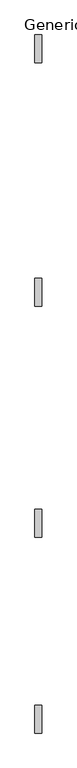
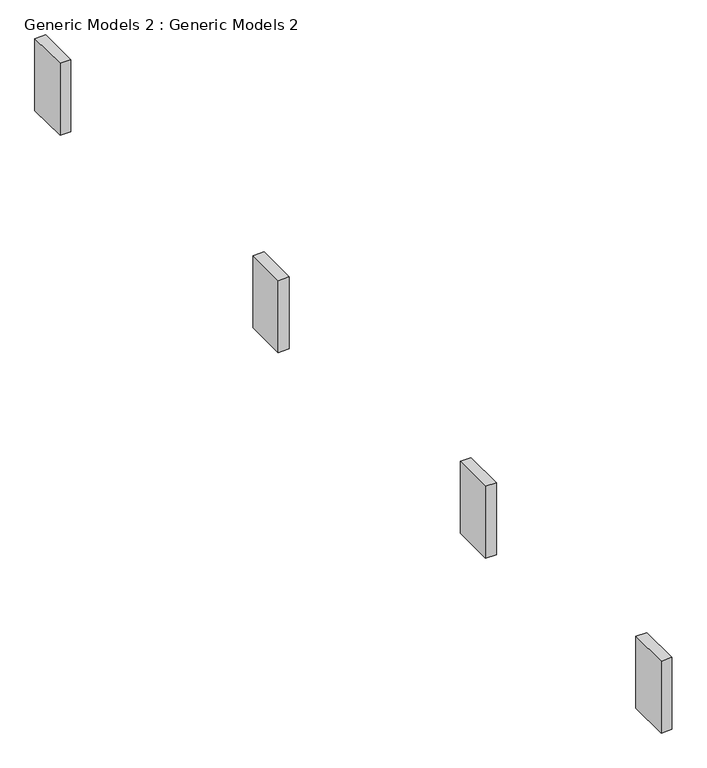
"""IFC4 building model written with IfcOpenShell, lengths in millimetres: proxy geometry, Generic Models 2 : Generic Models 2."""

from ifc_helpers import new_model, si_unit, frame, origin, place, context, project, spatial, polyline, outline, extrude, source, transform, mapped, element, save


def generic_models_2_generic_models_2_0c6c8571(model_context):
    return source(origin(), model_context, "Body", "SweptSolid", [
        extrude(outline(polyline([(-6761.5977342, -7156.2178788), (-6761.5977342, -6546.6178788), (-6609.1977342, -6546.6178788), (-6609.1977342, -7156.2178788), (-6761.5977342, -7156.2178788)])), frame((0.0, 0.0, 265.029607), z_axis=(0.0, 0.0, 1.0), x_axis=(1.0, 0.0, 0.0)), (0.0, 0.0, 1.0), 1066.8),
        extrude(outline(polyline([(-6761.5977342, -2889.0178788), (-6761.5977342, -2279.4178788), (-6609.1977342, -2279.4178788), (-6609.1977342, -2889.0178788), (-6761.5977342, -2889.0178788)])), frame((0.0, 0.0, 265.029607), z_axis=(0.0, 0.0, 1.0), x_axis=(1.0, 0.0, 0.0)), (0.0, 0.0, 1.0), 1066.8),
        extrude(outline(polyline([(-6761.5977342, 2140.1821212), (-6761.5977342, 2749.7821212), (-6609.1977342, 2749.7821212), (-6609.1977342, 2140.1821212), (-6761.5977342, 2140.1821212)])), frame((0.0, 0.0, 265.029607), z_axis=(0.0, 0.0, 1.0), x_axis=(1.0, 0.0, 0.0)), (0.0, 0.0, 1.0), 1066.8),
        extrude(outline(polyline([(-6761.5977342, 7441.8690558), (-6761.5977342, 8051.4690558), (-6609.1977342, 8051.4690558), (-6609.1977342, 7441.8690558), (-6761.5977342, 7441.8690558)])), frame((0.0, 0.0, 265.029607), z_axis=(0.0, 0.0, 1.0), x_axis=(1.0, 0.0, 0.0)), (0.0, 0.0, 1.0), 1066.8),
    ])


if __name__ == "__main__":
    model = new_model("IFC4")
    model_context = context("Model", 3, world=origin())
    ifc_project = project(units=[si_unit("LENGTHUNIT", "METRE", prefix="MILLI")], contexts=[model_context])
    site = spatial("IfcSite", under=ifc_project)
    building = spatial("IfcBuilding", under=site)
    placement = place(None, origin())
    generic_models_2_generic_models_2_shape = generic_models_2_generic_models_2_0c6c8571(model_context)
    element("IfcBuildingElementProxy", 1, Name="Generic Models 2 : Generic Models 2", ObjectType="Generic Models 2 : Generic Models 2", at=placement, inside=building, context=model_context, shape_type="MappedRepresentation", body=[
        mapped(generic_models_2_generic_models_2_shape, transform((0.0, 0.0, 0.0), x_axis=(1.0, 0.0, 0.0), y_axis=(0.0, 1.0, 0.0), z_axis=(0.0, 0.0, 1.0))),
    ])
    save(model, "model.ifc")

# Revit data of these elements
# Element 1 (IfcBuildingElementProxy, "Generic Models 2 : Generic Models 2")
#   Materials on its faces: "legs"
# Materials
#   "legs": colour RGB 90 73 37, transparency 0, Cost = 0
